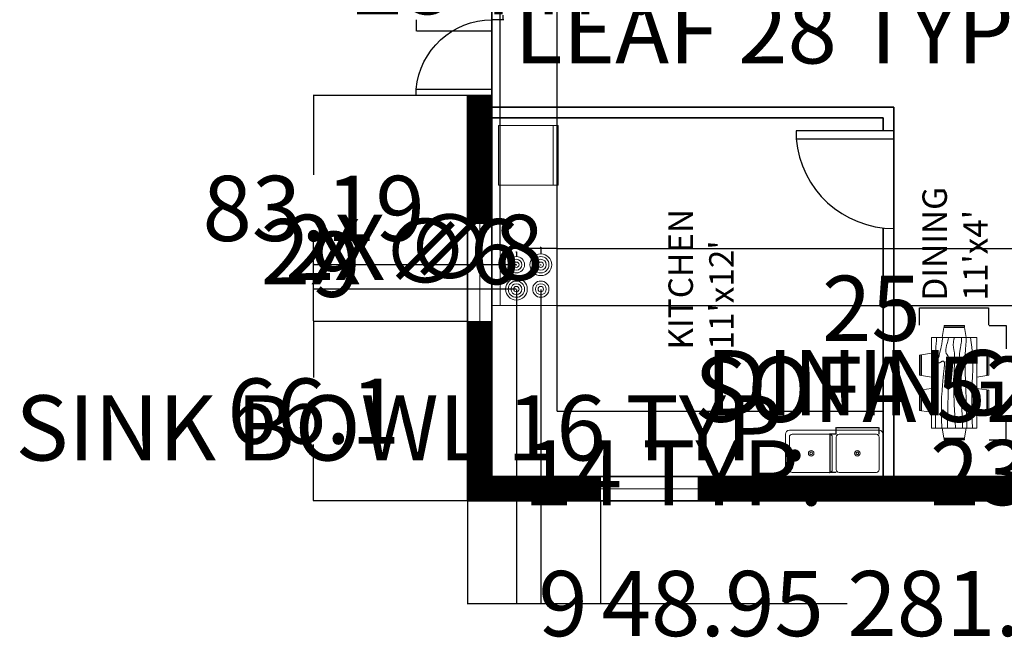
# Model space of a CAD drawing. Units: inches. Extents: x -1226 to 4538, y -998 to 1029.
# Tile 1 of 5: x -1226 to -864, y -998 to -767. Entities that reach past the tile are written whole.
import ezdxf

# ---------------------------------------------------------------- set-up
doc = ezdxf.new("R2010")
doc.units = ezdxf.units.IN
doc.header["$MEASUREMENT"] = 0
for name, color, linetype, lineweight in [('A-ANNO-DIMS', 2, 'Continuous', 18), ('A-AREA-IDEN', 7, 'Continuous', 18), ('A-DOOR', 4, 'Continuous', 25), ('A-EQPM', 8, 'Continuous', 18), ('A-FLOR-CASE', 8, 'Continuous', 25), ('A-FLOR-FIXT', 9, 'Continuous', 18), ('A-FURN', 8, 'Continuous', 18), ('A-GLAZ', 3, 'Continuous', 18), ('A-WALL', 7, 'Continuous', 35), ('A-WALL-PATT', 1, 'Continuous', 13)]:
    doc.layers.add(name, color=color, linetype=linetype, lineweight=lineweight)
doc.styles.get("Standard").update_dxf_attribs({"font": 'arial.ttf'})
doc.dimstyles.get("Standard").update_dxf_attribs({"dimtxt": 24, "dimasz": 0.18, "dimexe": 0.18, "dimexo": 0.0625, "dimgap": 0.09, "dimtad": 0, "dimtih": 1, "dimtoh": 1, "dimdec": 0, "dimzin": 0, "dimdsep": 46, "dimlunit": 4, "dimtxsty": 'Standard', "dimcen": 0.09, "dimadec": 0, "dimazin": 0, "dimtfac": 1, "dimtdec": 0, "dimtofl": 0, "dimtmove": 0, "dimatfit": 3, "dimfxl": 1, "dimtolj": 1, "dimtzin": 0, "dimarcsym": 0})

# ---------------------------------------------------------------- blocks, each defined once
blk = doc.blocks.new('Dining Set - 36 x 72 in.')
for p, q in [((-22.2343, 26.00059), (-23.4847, 17.99762)), ((-22.2304, 26), (-5.7608, 26)), ((-22, 27.5), (-22.1562, 26.50042)), ((-5.8416, 26.5), (-22.1534, 26.5)), ((-22, 27.5), (-6, 27.5)), ((-5.8437, 26.49966), (-6, 27.5)), ((-4.5152, 17.99762), (-5.7655, 25.99926)), ((5.7657, 26.00059), (4.5153, 17.99762)), ((5.7696, 26), (22.2392, 26)), ((6, 27.5), (5.8438, 26.50042)), ((22.1584, 26.5), (5.8466, 26.5)), ((6, 27.5), (22, 27.5)), ((22.1563, 26.49966), (22, 27.5)), ((23.4848, 17.99762), (22.2345, 25.99926)), ((36, 18), (-36, 18)), ((-36, 18), (-36, -18)), ((36, -18), (36, 18)), ((-45.5, 8), (-44.5004, 8.15617)), ((-45.5, 8), (-45.5, -8)), ((-44.5, -8.15843), (-44.5, 8.15338)), ((-44.0006, 8.23428), (-35.9976, 9.48474)), ((-44, 8.23041), (-44, -8.23915)), ((44.0006, 8.23428), (35.9976, 9.48474)), ((44, 8.23041), (44, -8.23915)), ((44.5, -8.15843), (44.5, 8.15338)), ((45.5, 8), (44.5005, 8.15617)), ((45.5, 8), (45.5, -8)), ((-44.4997, -8.15631), (-45.5, -8)), ((-35.9976, -9.48476), (-43.9993, -8.2345)), ((35.9976, -9.48476), (43.9993, -8.2345)), ((44.4997, -8.15631), (45.5, -8)), ((-36, -18), (36, -18)), ((-22.2343, -26.0006), (-23.4847, -17.99762)), ((-4.5152, -17.99762), (-5.7655, -25.99928)), ((5.7657, -26.0006), (4.5153, -17.99762)), ((23.4848, -17.99762), (22.2345, -25.99928)), ((-22.2304, -26), (-5.7608, -26)), ((-22, -27.5), (-22.1562, -26.50044)), ((-5.8416, -26.5), (-22.1534, -26.5)), ((-22, -27.5), (-6, -27.5)), ((-5.8437, -26.49967), (-6, -27.5)), ((5.7696, -26), (22.2392, -26)), ((6, -27.5), (5.8438, -26.50044)), ((22.1584, -26.5), (5.8466, -26.5)), ((6, -27.5), (22, -27.5)), ((22.1563, -26.49967), (22, -27.5))]:
    blk.add_line(p, q)
for points in [[(-36, 15), (-31.1772, 14.97754), (-26.8079, 14.91406), (-22.8538, 14.81543), (-19.276, 14.6875), (-16.0362, 14.53613), (-13.0957, 14.36718), (-10.4159, 14.18652), (-7.9583, 14), (-5.6904, 13.81315), (-3.6035, 13.63021), (-1.6954, 13.45508), (0.0365, 13.29166), (1.5945, 13.14388), (2.9811, 13.01562), (4.1988, 12.9108), (5.25, 12.83333), (6.1393, 12.78613), (6.8802, 12.76823), (7.4883, 12.77767), (7.9792, 12.8125), (8.3685, 12.87077), (8.6719, 12.95052), (8.9049, 13.0498), (9.0833, 13.16666), (9.2205, 13.29899), (9.3216, 13.44401), (9.3895, 13.59879), (9.4271, 13.76041), (9.4373, 13.92594), (9.4232, 14.09245), (9.3875, 14.257), (9.3333, 14.41666), (9.2638, 14.56917), (9.1836, 14.71484), (9.0975, 14.85465), (9.0104, 14.98958), (8.9272, 15.1206), (8.8529, 15.2487), (8.7922, 15.37483), (8.75, 15.5), (8.7305, 15.62467), (8.7344, 15.74739), (8.7617, 15.86621), (8.8125, 15.97916), (8.8867, 16.08431), (8.9844, 16.17968), (9.1055, 16.26334), (9.25, 16.33333), (9.4189, 16.38802), (9.6172, 16.42708), (9.8506, 16.45052), (10.125, 16.45833), (10.4463, 16.45052), (10.8203, 16.42708), (11.2529, 16.38802), (11.75, 16.33333), (12.3184, 16.26318), (12.9694, 16.17838), (13.7151, 16.07991), (14.5677, 15.96875), (15.5395, 15.84586), (16.6426, 15.71224), (17.8893, 15.56884), (19.2917, 15.41666), (20.859, 15.25667), (22.5879, 15.08984), (24.4721, 14.91715), (26.5052, 14.73958), (28.6809, 14.5581), (30.9929, 14.3737), (33.4347, 14.18733), (36, 14)], [(-36, 10), (-28.9766, 10.14274), (-23.1725, 10.20442), (-18.4241, 10.19775), (-14.5677, 10.13541), (-11.4399, 10.03011), (-8.877, 9.89453), (-6.7154, 9.74137), (-4.7917, 9.58333), (-2.9698, 9.43082), (-1.2246, 9.28515), (0.4415, 9.14534), (2.026, 9.01041), (3.5266, 8.87939), (4.9408, 8.7513), (6.266, 8.62516), (7.5, 8.5), (8.6411, 8.37549), (9.6914, 8.2539), (10.6538, 8.13818), (11.5312, 8.03125), (12.3267, 7.93603), (13.043, 7.85547), (13.6831, 7.79248), (14.25, 7.75), (14.7471, 7.7303), (15.1797, 7.73307), (15.5537, 7.75732), (15.875, 7.80208), (16.1494, 7.86637), (16.3828, 7.94922), (16.5811, 8.04964), (16.75, 8.16666), (16.8944, 8.29915), (17.0143, 8.44531), (17.1089, 8.60319), (17.1771, 8.77083), (17.218, 8.94629), (17.2305, 9.1276), (17.2137, 9.31282), (17.1667, 9.5), (17.0895, 9.6875), (16.987, 9.875), (16.8649, 10.0625), (16.7292, 10.25), (16.5856, 10.4375), (16.4401, 10.625), (16.2985, 10.8125), (16.1667, 11), (16.05, 11.18733), (15.9518, 11.3737), (15.8752, 11.5581), (15.8229, 11.73958), (15.798, 11.91715), (15.8034, 12.08984), (15.842, 12.25667), (15.9167, 12.41666), (16.0295, 12.56836), (16.1784, 12.70833), (16.3605, 12.83268), (16.5729, 12.9375), (16.8127, 13.01888), (17.0768, 13.07291), (17.3625, 13.0957), (17.6667, 13.08333), (17.9894, 13.03312), (18.3418, 12.94726), (18.7382, 12.82918), (19.1927, 12.68229), (19.7195, 12.51001), (20.3327, 12.31575), (21.0465, 12.10294), (21.875, 11.875), (22.8357, 11.63354), (23.959, 11.37304), (25.2786, 11.08618), (26.8282, 10.76562), (28.6414, 10.40405), (30.752, 9.99414), (33.1936, 9.52856), (36, 9)], [(-36, 5.5), (-30.7157, 5.3348), (-26.069, 5.20963), (-21.9946, 5.11767), (-18.4271, 5.05208), (-15.3009, 5.00602), (-12.5508, 4.97265), (-10.1112, 4.94515), (-7.9167, 4.91666), (-5.909, 4.88167), (-4.0586, 4.83984), (-2.3429, 4.79215), (-0.7396, 4.73958), (0.7739, 4.6831), (2.22, 4.6237), (3.6213, 4.56233), (5, 4.5), (6.373, 4.43782), (7.7344, 4.3776), (9.0723, 4.32129), (10.375, 4.27083), (11.6309, 4.22819), (12.8281, 4.19531), (13.9551, 4.17415), (15, 4.16666), (15.954, 4.17448), (16.819, 4.19791), (17.6001, 4.23698), (18.3021, 4.29166), (18.9299, 4.36198), (19.4883, 4.44791), (19.9823, 4.54948), (20.4167, 4.66666), (20.7969, 4.79899), (21.1302, 4.94401), (21.4245, 5.09879), (21.6875, 5.26041), (21.9271, 5.42594), (22.1511, 5.59245), (22.3672, 5.757), (22.5834, 5.91666), (22.8065, 6.06868), (23.0404, 6.21093), (23.2879, 6.34147), (23.5521, 6.45833), (23.8358, 6.55957), (24.142, 6.64323), (24.4735, 6.70735), (24.8334, 6.75), (25.2235, 6.76969), (25.642, 6.76692), (26.0858, 6.74267), (26.5521, 6.69791), (27.0379, 6.63362), (27.5404, 6.55078), (28.0565, 6.45036), (28.5834, 6.33333), (29.1242, 6.19987), (29.7071, 6.04687), (30.3661, 5.87044), (31.1354, 5.66666), (32.0493, 5.43164), (33.142, 5.16146), (34.4475, 4.85221), (36, 4.5)], [(-36, -1), (-30.7915, -0.6591), (-26.0195, -0.38216), (-21.6519, -0.16284), (-17.6563, 0.00521), (-14.0005, 0.12833), (-10.6523, 0.21289), (-7.5796, 0.26522), (-4.75, 0.29166), (-2.134, 0.29793), (0.2878, 0.28711), (2.5317, 0.26163), (4.6146, 0.22396), (6.5529, 0.17651), (8.3633, 0.12174), (10.0623, 0.06209), (11.6667, 0), (13.1899, -0.06201), (14.6341, -0.1211), (15.9982, -0.17432), (17.2813, -0.21875), (18.4823, -0.25147), (19.6003, -0.26953), (20.6343, -0.27002), (21.5834, -0.25), (22.4481, -0.20768), (23.2357, -0.14584), (23.9549, -0.06836), (24.6146, 0.02083), (25.2235, 0.11784), (25.7904, 0.21875), (26.3241, 0.31966), (26.8334, 0.41666), (27.3265, 0.50618), (27.8099, 0.58593), (28.2894, 0.65397), (28.7709, 0.70833), (29.2601, 0.74707), (29.763, 0.76823), (30.2855, 0.76985), (30.8334, 0.75), (31.4088, 0.70784), (31.9994, 0.64713), (32.589, 0.57275), (33.1615, 0.48958), (33.7008, 0.4025), (34.1908, 0.3164), (34.6153, 0.23616), (34.9584, 0.16666), (35.2099, 0.11165), (35.3848, 0.07031), (35.504, 0.04069), (35.5886, 0.02083), (35.6594, 0.00879), (35.7377, 0.0026), (35.8442, 0.00032), (36, 0)], [(-36, -6.5), (-27.1843, -6.31267), (-20.084, -6.1263), (-14.469, -5.9419), (-10.1094, -5.76042), (-6.7752, -5.58285), (-4.2363, -5.41016), (-2.2629, -5.24333), (-0.625, -5.08334), (0.8708, -4.93099), (2.2715, -4.78646), (3.5872, -4.64974), (4.8281, -4.52084), (6.0046, -4.39974), (7.127, -4.28646), (8.2053, -4.18099), (9.25, -4.08334), (10.2705, -3.99382), (11.2734, -3.91407), (12.2647, -3.84603), (13.25, -3.79167), (14.2354, -3.75293), (15.2266, -3.73177), (16.2295, -3.73015), (17.25, -3.75), (18.2912, -3.79248), (19.3451, -3.85547), (20.4009, -3.93604), (21.4479, -4.03125), (22.4754, -4.13819), (23.4727, -4.25391), (24.4289, -4.37549), (25.3334, -4.5), (26.1785, -4.62492), (26.9694, -4.74935), (27.7145, -4.87281), (28.4219, -4.99479), (29.1, -5.11483), (29.7572, -5.23242), (30.4016, -5.34709), (31.0417, -5.45834), (31.6837, -5.56437), (32.3262, -5.65821), (32.9658, -5.73153), (33.599, -5.77604), (34.2224, -5.78345), (34.8327, -5.74545), (35.4264, -5.65373), (36, -5.5)], [(-36, -10), (-26.4022, -9.81299), (-18.4675, -9.62891), (-11.9839, -9.45069), (-6.7396, -9.28125), (-2.5226, -9.12354), (0.8789, -8.98047), (3.6769, -8.85498), (6.0833, -8.75), (8.2767, -8.66765), (10.3021, -8.60677), (12.1712, -8.56543), (13.8958, -8.54167), (15.4876, -8.53353), (16.9583, -8.53907), (18.3197, -8.55632), (19.5834, -8.58334), (20.7616, -8.61841), (21.8685, -8.66081), (22.9188, -8.71004), (23.9271, -8.76563), (24.9081, -8.82707), (25.8763, -8.89388), (26.8465, -8.96558), (27.8334, -9.04167), (28.8474, -9.12118), (29.8828, -9.20117), (30.93, -9.27824), (31.9792, -9.34896), (33.0205, -9.40991), (34.0443, -9.45768), (35.0407, -9.48885), (36, -9.5)], [(-36, -14.5), (-30.0881, -14.33513), (-25.0332, -14.21224), (-20.7312, -14.12647), (-17.0781, -14.07292), (-13.97, -14.04671), (-11.3027, -14.04297), (-8.9724, -14.05681), (-6.875, -14.08334), (-4.9224, -14.11833), (-3.0905, -14.16016), (-1.3709, -14.20785), (0.2448, -14.26042), (1.7647, -14.3169), (3.1973, -14.3763), (4.5507, -14.43767), (5.8333, -14.5), (7.0554, -14.5621), (8.235, -14.62175), (9.3922, -14.67652), (10.5469, -14.72396), (11.7192, -14.76164), (12.929, -14.78711), (14.1965, -14.79794), (15.5417, -14.79167), (16.9933, -14.76424), (18.6152, -14.70508), (20.4804, -14.60197), (22.6615, -14.44271), (25.2312, -14.21509), (28.2624, -13.9069), (31.8277, -13.50594), (36, -13)]]:
    blk.add_lwpolyline(points)
blk = doc.blocks.new('DOOR-SWING-36')
for p, q in [((36, 36), (0, 36)), ((0, 36), (0, 33)), ((0, 33), (36, 33)), ((36, 33), (36, 36))]:
    blk.add_line(p, q)
blk.add_arc((36, 36.14), 36.14, 184.9791, 270)
blk = doc.blocks.new('DOOR-SWING-NARROW')
for p, q in [((27.84, 27.84), (0, 27.84)), ((0, 27.84), (0, 25.52)), ((0, 25.52), (27.84, 25.52)), ((27.84, 25.52), (27.84, 27.84))]:
    blk.add_line(p, q)
blk.add_arc((27.84, 27.94), 27.94, 184.9791, 270)
blk = doc.blocks.new('WIN-36')
for p, q in [((0, 36), (9, 36)), ((4.5, 0), (4.5, 36)), ((0, 0), (9, 0))]:
    blk.add_line(p, q)
blk = doc.blocks.new('SINK-BOWL-STANDARD')
blk.add_line((15.75, 1), (15.75, 13))
for points in [[(0, 1), (0, 13)], [(1, 14), (14.75, 14)], [(14.75, 0), (1, 0)]]:
    blk.add_lwpolyline(points)
for radius in [1, 0.5]:
    blk.add_circle((8, 7), radius)
for centre, start, end in [((1, 13), 90, 180), ((14.75, 13), 0, 90), ((1, 1), 180, 270), ((14.75, 1), 270, 0)]:
    blk.add_arc(centre, 1, start, end)
blk = doc.blocks.new('BURNER-6IN')
for radius in [3, 2, 1]:
    blk.add_circle((3, 3), radius)
blk = doc.blocks.new('BURNER-8IN')
for radius in [4, 3, 2, 1]:
    blk.add_circle((4, 4), radius)
blk = doc.blocks.new('*D28')
at = {"layer": 'A-ANNO-DIMS', "color": 0, "lineweight": -2, "transparency": 16777216}
for p, q in [((-1080.03, -767.33), (-1080.03, -771.62)), ((-1052.19, -767.33), (-1052.19, -771.62)), ((-1079.85, -771.44), (-1052.37, -771.44)), ((-1052.19, -771.44), (-1052.01, -771.44))]:
    blk.add_line(p, q, dxfattribs=at)
at = {"layer": 'A-ANNO-DIMS', "color": 0, "transparency": 16777216}
for points in [[(-1079.85, -771.41), (-1079.85, -771.47), (-1080.03, -771.44)], [(-1052.37, -771.41), (-1052.37, -771.47), (-1052.19, -771.44)]]:
    blk.add_solid(points, dxfattribs=at)
at = {"layer": 'Defpoints', "color": 0, "transparency": 16777216}
for p in [(-1080.03, -767.26), (-1052.19, -767.26), (-1052.19, -771.44)]:
    blk.add_point(p, dxfattribs=at)
at = {"layer": 'A-ANNO-DIMS', "color": 0, "transparency": 16777216, "insert": (-947.45, -771.44), "char_height": 24, "attachment_point": 5}
blk.add_mtext('\\A1;LEAF 28 TYP.', dxfattribs=at)
blk = doc.blocks.new('*D29')
at = {"layer": 'A-ANNO-DIMS', "color": 0, "lineweight": -2, "transparency": 16777216}
for p, q in [((-1052.13, -739.42), (-1047.83, -739.42)), ((-1048.01, -739.6), (-1048.01, -741)), ((-1052.13, -767.26), (-1047.83, -767.26)), ((-1048.01, -767.08), (-1048.01, -765.69))]:
    blk.add_line(p, q, dxfattribs=at)
at = {"layer": 'A-ANNO-DIMS', "color": 0, "transparency": 16777216}
for points in [[(-1048.04, -739.6), (-1047.98, -739.6), (-1048.01, -739.42)], [(-1048.04, -767.08), (-1047.98, -767.08), (-1048.01, -767.26)]]:
    blk.add_solid(points, dxfattribs=at)
at = {"layer": 'Defpoints', "color": 0, "transparency": 16777216}
for p in [(-1052.19, -739.42), (-1048.01, -739.42), (-1052.19, -767.26)]:
    blk.add_point(p, dxfattribs=at)
at = {"layer": 'A-ANNO-DIMS', "color": 0, "transparency": 16777216, "insert": (-1048.01, -753.34), "char_height": 24, "attachment_point": 5}
blk.add_mtext('\\A1;28 TYP.', dxfattribs=at)
blk = doc.blocks.new('*D34')
at = {"layer": 'A-ANNO-DIMS', "color": 0, "lineweight": -2, "transparency": 16777216}
for p, q in [((-768.95, -903.42), (-769.13, -903.42)), ((-768.95, -911.16), (-768.95, -903.24)), ((-717.1, -903.42), (-768.77, -903.42)), ((-716.92, -911.16), (-716.92, -903.24))]:
    blk.add_line(p, q, dxfattribs=at)
at = {"layer": 'A-ANNO-DIMS', "color": 0, "transparency": 16777216}
for points in [[(-768.77, -903.39), (-768.77, -903.45), (-768.95, -903.42)], [(-717.1, -903.39), (-717.1, -903.45), (-716.92, -903.42)]]:
    blk.add_solid(points, dxfattribs=at)
at = {"layer": 'Defpoints', "color": 0, "transparency": 16777216}
for p in [(-768.95, -903.42), (-768.95, -911.22), (-716.92, -911.22)]:
    blk.add_point(p, dxfattribs=at)
at = {"layer": 'A-ANNO-DIMS', "color": 0, "transparency": 16777216, "insert": (-877.88, -903.42), "char_height": 24, "attachment_point": 5}
blk.add_mtext('\\A1;SOFA 52 TYP.', dxfattribs=at)
blk = doc.blocks.new('*D35')
at = {"layer": 'A-ANNO-DIMS', "color": 0, "lineweight": -2, "transparency": 16777216}
for p, q in [((-769.01, -911.22), (-776.94, -911.22)), ((-776.76, -911.4), (-776.76, -933.75)), ((-769.01, -933.93), (-776.94, -933.93)), ((-776.76, -934.11), (-776.94, -934.11)), ((-776.76, -933.93), (-776.76, -934.11))]:
    blk.add_line(p, q, dxfattribs=at)
at = {"layer": 'A-ANNO-DIMS', "color": 0, "transparency": 16777216}
for points in [[(-776.79, -911.4), (-776.73, -911.4), (-776.76, -911.22)], [(-776.79, -933.75), (-776.73, -933.75), (-776.76, -933.93)]]:
    blk.add_solid(points, dxfattribs=at)
at = {"layer": 'Defpoints', "color": 0, "transparency": 16777216}
for p in [(-768.95, -911.22), (-776.76, -933.93), (-768.95, -933.93)]:
    blk.add_point(p, dxfattribs=at)
at = {"layer": 'A-ANNO-DIMS', "color": 0, "transparency": 16777216, "insert": (-835.64, -934.11), "char_height": 24, "attachment_point": 5}
blk.add_mtext('\\A1;23 TYP.', dxfattribs=at)
blk = doc.blocks.new('*D40')
at = {"layer": 'A-ANNO-DIMS', "color": 0, "lineweight": -2, "transparency": 16777216}
for p, q in [((-925.4, -917.65), (-925.58, -917.65)), ((-925.4, -919.95), (-925.4, -917.47)), ((-909.83, -917.65), (-925.22, -917.65)), ((-909.65, -919.95), (-909.65, -917.47))]:
    blk.add_line(p, q, dxfattribs=at)
at = {"layer": 'A-ANNO-DIMS', "color": 0, "transparency": 16777216}
for points in [[(-925.22, -917.62), (-925.22, -917.68), (-925.4, -917.65)], [(-909.83, -917.62), (-909.83, -917.68), (-909.65, -917.65)]]:
    blk.add_solid(points, dxfattribs=at)
at = {"layer": 'Defpoints', "color": 0, "transparency": 16777216}
for p in [(-925.4, -917.65), (-925.4, -920.02), (-909.65, -920.02)]:
    blk.add_point(p, dxfattribs=at)
at = {"layer": 'A-ANNO-DIMS', "color": 0, "transparency": 16777216, "insert": (-1081.83, -917.65), "char_height": 24, "attachment_point": 5}
blk.add_mtext('\\A1;SINK BOWL 16 TYP.', dxfattribs=at)
blk = doc.blocks.new('*D41')
at = {"layer": 'A-ANNO-DIMS', "color": 0, "lineweight": -2, "transparency": 16777216}
for p, q in [((-925.46, -920.02), (-927.94, -920.02)), ((-927.76, -920.2), (-927.76, -933.84)), ((-925.46, -934.02), (-927.94, -934.02)), ((-927.76, -934.2), (-927.94, -934.2)), ((-927.76, -934.02), (-927.76, -934.2))]:
    blk.add_line(p, q, dxfattribs=at)
at = {"layer": 'A-ANNO-DIMS', "color": 0, "transparency": 16777216}
for points in [[(-927.79, -920.2), (-927.73, -920.2), (-927.76, -920.02)], [(-927.79, -933.84), (-927.73, -933.84), (-927.76, -934.02)]]:
    blk.add_solid(points, dxfattribs=at)
at = {"layer": 'Defpoints', "color": 0, "transparency": 16777216}
for p in [(-925.4, -920.02), (-927.76, -934.02), (-925.4, -934.02)]:
    blk.add_point(p, dxfattribs=at)
at = {"layer": 'A-ANNO-DIMS', "color": 0, "transparency": 16777216, "insert": (-985.31, -934.2), "char_height": 24, "attachment_point": 5}
blk.add_mtext('\\A1;14 TYP.', dxfattribs=at)
blk = doc.blocks.new('*D46')
at = {"layer": 'A-ANNO-DIMS', "color": 0, "lineweight": -2, "transparency": 16777216}
for p, q in [((-869.17, -879.93), (-862.73, -879.93)), ((-862.91, -880.11), (-862.91, -888.51)), ((-862.91, -921.91), (-862.91, -913.51)), ((-869.17, -922.09), (-862.73, -922.09))]:
    blk.add_line(p, q, dxfattribs=at)
at = {"layer": 'A-ANNO-DIMS', "color": 0, "transparency": 16777216}
for points in [[(-862.94, -880.11), (-862.88, -880.11), (-862.91, -879.93)], [(-862.94, -921.91), (-862.88, -921.91), (-862.91, -922.09)]]:
    blk.add_solid(points, dxfattribs=at)
at = {"layer": 'Defpoints', "color": 0, "transparency": 16777216}
for p in [(-869.23, -879.93), (-862.91, -879.93), (-869.23, -922.09)]:
    blk.add_point(p, dxfattribs=at)
at = {"layer": 'A-ANNO-DIMS', "color": 0, "transparency": 16777216, "insert": (-862.91, -901.01), "char_height": 24, "attachment_point": 5}
blk.add_mtext('\\A1;DINING SET 42', dxfattribs=at)
blk = doc.blocks.new('*D47')
at = {"layer": 'A-ANNO-DIMS', "color": 0, "lineweight": -2, "transparency": 16777216}
for p, q in [((-894.72, -879.87), (-894.72, -873.43)), ((-869.23, -879.87), (-869.23, -873.43)), ((-894.72, -873.61), (-894.9, -873.61)), ((-869.41, -873.61), (-894.54, -873.61))]:
    blk.add_line(p, q, dxfattribs=at)
at = {"layer": 'A-ANNO-DIMS', "color": 0, "transparency": 16777216}
for points in [[(-894.54, -873.58), (-894.54, -873.64), (-894.72, -873.61)], [(-869.41, -873.58), (-869.41, -873.64), (-869.23, -873.61)]]:
    blk.add_solid(points, dxfattribs=at)
at = {"layer": 'Defpoints', "color": 0, "transparency": 16777216}
for p in [(-894.72, -873.61), (-894.72, -879.93), (-869.23, -879.93)]:
    blk.add_point(p, dxfattribs=at)
at = {"layer": 'A-ANNO-DIMS', "color": 0, "transparency": 16777216, "insert": (-912.47, -873.61), "char_height": 24, "attachment_point": 5}
blk.add_mtext('\\A1;25', dxfattribs=at)
blk = doc.blocks.new('*D56')
at = {"layer": 'A-ANNO-DIMS', "color": 0, "lineweight": -2, "transparency": 16777216}
for p, q in [((-1061.17, -944.59), (-1061.17, -982.51)), ((-1012.21, -944.64), (-1012.21, -982.51)), ((-1060.99, -982.33), (-1012.39, -982.33)), ((-1012.21, -982.33), (-1012.03, -982.33))]:
    blk.add_line(p, q, dxfattribs=at)
at = {"layer": 'A-ANNO-DIMS', "color": 0, "transparency": 16777216}
for points in [[(-1060.99, -982.3), (-1060.99, -982.36), (-1061.17, -982.33)], [(-1012.39, -982.3), (-1012.39, -982.36), (-1012.21, -982.33)]]:
    blk.add_solid(points, dxfattribs=at)
at = {"layer": 'Defpoints', "color": 0, "transparency": 16777216}
for p in [(-1061.17, -944.53), (-1012.21, -944.57), (-1012.21, -982.33)]:
    blk.add_point(p, dxfattribs=at)
at = {"layer": 'A-ANNO-DIMS', "color": 0, "transparency": 16777216, "insert": (-970.88, -982.33), "char_height": 24, "attachment_point": 5}
blk.add_mtext('\\A1;48.95', dxfattribs=at)
blk = doc.blocks.new('*D57')
at = {"layer": 'A-ANNO-DIMS', "color": 0, "lineweight": -2, "transparency": 16777216}
for p, q in [((-1012.21, -944.64), (-1012.21, -982.51)), ((-730.47, -944.64), (-730.47, -982.51)), ((-1012.03, -982.33), (-921.41, -982.33)), ((-730.65, -982.33), (-821.28, -982.33))]:
    blk.add_line(p, q, dxfattribs=at)
at = {"layer": 'A-ANNO-DIMS', "color": 0, "transparency": 16777216}
for points in [[(-1012.03, -982.3), (-1012.03, -982.36), (-1012.21, -982.33)], [(-730.65, -982.3), (-730.65, -982.36), (-730.47, -982.33)]]:
    blk.add_solid(points, dxfattribs=at)
at = {"layer": 'Defpoints', "color": 0, "transparency": 16777216}
for p in [(-1012.21, -944.57), (-730.47, -944.58), (-730.47, -982.33)]:
    blk.add_point(p, dxfattribs=at)
at = {"layer": 'A-ANNO-DIMS', "color": 0, "transparency": 16777216, "insert": (-871.34, -982.33), "char_height": 24, "attachment_point": 5}
blk.add_mtext('\\A1;281.74', dxfattribs=at)
blk = doc.blocks.new('*D59')
at = {"layer": 'A-ANNO-DIMS', "color": 0, "lineweight": -2, "transparency": 16777216}
for p, q in [((-1061.14, -878.43), (-1117.96, -878.43)), ((-1117.78, -878.61), (-1117.78, -899.13)), ((-1117.78, -944.35), (-1117.78, -923.82)), ((-1061.23, -944.53), (-1117.96, -944.53))]:
    blk.add_line(p, q, dxfattribs=at)
at = {"layer": 'A-ANNO-DIMS', "color": 0, "transparency": 16777216}
for points in [[(-1117.81, -878.61), (-1117.75, -878.61), (-1117.78, -878.43)], [(-1117.81, -944.35), (-1117.75, -944.35), (-1117.78, -944.53)]]:
    blk.add_solid(points, dxfattribs=at)
at = {"layer": 'Defpoints', "color": 0, "transparency": 16777216}
for p in [(-1117.78, -878.43), (-1061.07, -878.43), (-1061.17, -944.53)]:
    blk.add_point(p, dxfattribs=at)
at = {"layer": 'A-ANNO-DIMS', "color": 0, "transparency": 16777216, "insert": (-1117.78, -911.48), "char_height": 24, "attachment_point": 5}
blk.add_mtext('\\A1;66.1', dxfattribs=at)
blk = doc.blocks.new('*D60')
at = {"layer": 'A-ANNO-DIMS', "color": 0, "lineweight": -2, "transparency": 16777216}
for p, q in [((-1061.23, -795.24), (-1117.96, -795.24)), ((-1117.78, -795.42), (-1117.78, -824.48)), ((-1117.78, -878.25), (-1117.78, -849.19)), ((-1061.14, -878.43), (-1117.96, -878.43))]:
    blk.add_line(p, q, dxfattribs=at)
at = {"layer": 'A-ANNO-DIMS', "color": 0, "transparency": 16777216}
for points in [[(-1117.81, -795.42), (-1117.75, -795.42), (-1117.78, -795.24)], [(-1117.81, -878.25), (-1117.75, -878.25), (-1117.78, -878.43)]]:
    blk.add_solid(points, dxfattribs=at)
at = {"layer": 'Defpoints', "color": 0, "transparency": 16777216}
for p in [(-1117.78, -795.24), (-1061.17, -795.24), (-1061.07, -878.43)]:
    blk.add_point(p, dxfattribs=at)
at = {"layer": 'A-ANNO-DIMS', "color": 0, "transparency": 16777216, "insert": (-1117.78, -836.83), "char_height": 24, "attachment_point": 5}
blk.add_mtext('\\A1;83.19', dxfattribs=at)
blk = doc.blocks.new('*D77')
at = {"layer": 'A-ANNO-DIMS', "color": 0, "lineweight": -2, "transparency": 16777216}
for p, q in [((-1049.16, -851.5), (-1049.16, -546.6)), ((-1048.98, -546.78), (-1028.34, -546.78)), ((-1028.16, -851.5), (-1028.16, -546.6)), ((-1028.16, -546.78), (-1027.98, -546.78))]:
    blk.add_line(p, q, dxfattribs=at)
at = {"layer": 'A-ANNO-DIMS', "color": 0, "transparency": 16777216}
for points in [[(-1048.98, -546.75), (-1048.98, -546.81), (-1049.16, -546.78)], [(-1028.34, -546.75), (-1028.34, -546.81), (-1028.16, -546.78)]]:
    blk.add_solid(points, dxfattribs=at)
at = {"layer": 'Defpoints', "color": 0, "transparency": 16777216}
for p in [(-1028.16, -546.78), (-1049.16, -851.56), (-1028.16, -851.56)]:
    blk.add_point(p, dxfattribs=at)
at = {"layer": 'A-ANNO-DIMS', "color": 0, "transparency": 16777216, "insert": (-1012.81, -546.78), "char_height": 24, "attachment_point": 5}
blk.add_mtext('\\A1;21', dxfattribs=at)
blk = doc.blocks.new('*D78')
at = {"layer": 'A-ANNO-DIMS', "color": 0, "lineweight": -2, "transparency": 16777216}
for p, q in [((-1028.09, -851.56), (-401.24, -851.56)), ((-401.42, -851.74), (-401.42, -872.38)), ((-1028.09, -872.56), (-401.24, -872.56)), ((-401.42, -872.74), (-401.6, -872.74)), ((-401.42, -872.56), (-401.42, -872.74))]:
    blk.add_line(p, q, dxfattribs=at)
at = {"layer": 'A-ANNO-DIMS', "color": 0, "transparency": 16777216}
for points in [[(-401.45, -851.74), (-401.39, -851.74), (-401.42, -851.56)], [(-401.45, -872.38), (-401.39, -872.38), (-401.42, -872.56)]]:
    blk.add_solid(points, dxfattribs=at)
at = {"layer": 'Defpoints', "color": 0, "transparency": 16777216}
for p in [(-1028.16, -851.56), (-1028.16, -872.56), (-401.42, -872.56)]:
    blk.add_point(p, dxfattribs=at)
at = {"layer": 'A-ANNO-DIMS', "color": 0, "transparency": 16777216, "insert": (-416.76, -872.74), "char_height": 24, "attachment_point": 5}
blk.add_mtext('\\A1;21', dxfattribs=at)
blk = doc.blocks.new('*D79')
at = {"layer": 'A-ANNO-DIMS', "color": 0, "lineweight": -2, "transparency": 16777216}
for p, q in [((-1043.16, -866.63), (-1043.16, -982.51)), ((-1034.16, -866.63), (-1034.16, -982.51)), ((-1042.98, -982.33), (-1034.34, -982.33)), ((-1034.16, -982.33), (-1033.98, -982.33))]:
    blk.add_line(p, q, dxfattribs=at)
at = {"layer": 'A-ANNO-DIMS', "color": 0, "transparency": 16777216}
for points in [[(-1042.98, -982.3), (-1042.98, -982.36), (-1043.16, -982.33)], [(-1034.34, -982.3), (-1034.34, -982.36), (-1034.16, -982.33)]]:
    blk.add_solid(points, dxfattribs=at)
at = {"layer": 'Defpoints', "color": 0, "transparency": 16777216}
for p in [(-1043.16, -866.56), (-1034.16, -866.56), (-1034.16, -982.33)]:
    blk.add_point(p, dxfattribs=at)
at = {"layer": 'A-ANNO-DIMS', "color": 0, "transparency": 16777216, "insert": (-1026, -982.33), "char_height": 24, "attachment_point": 5}
blk.add_mtext('\\A1;9', dxfattribs=at)
blk = doc.blocks.new('*D80')
at = {"layer": 'A-ANNO-DIMS', "color": 0, "lineweight": -2, "transparency": 16777216}
for p, q in [((-1043.22, -857.56), (-1117.96, -857.56)), ((-1117.78, -857.56), (-1117.78, -857.38)), ((-1117.78, -857.38), (-1117.6, -857.38)), ((-1117.78, -866.38), (-1117.78, -857.74)), ((-1043.22, -866.56), (-1117.96, -866.56))]:
    blk.add_line(p, q, dxfattribs=at)
at = {"layer": 'A-ANNO-DIMS', "color": 0, "transparency": 16777216}
for points in [[(-1117.81, -857.74), (-1117.75, -857.74), (-1117.78, -857.56)], [(-1117.81, -866.38), (-1117.75, -866.38), (-1117.78, -866.56)]]:
    blk.add_solid(points, dxfattribs=at)
at = {"layer": 'Defpoints', "color": 0, "transparency": 16777216}
for p in [(-1117.78, -857.56), (-1043.16, -857.56), (-1043.16, -866.56)]:
    blk.add_point(p, dxfattribs=at)
at = {"layer": 'A-ANNO-DIMS', "color": 0, "transparency": 16777216, "insert": (-1109.62, -857.38), "char_height": 24, "attachment_point": 5}
blk.add_mtext('\\A1;9', dxfattribs=at)
blk = doc.blocks.new('*D81')
at = {"layer": 'A-ANNO-DIMS', "color": 0, "lineweight": -2, "transparency": 16777216}
for p, q in [((-1043.34, -852.76), (-1043.16, -852.76)), ((-1043.16, -852.76), (-1043.16, -854.38)), ((-1043.25, -857.56), (-1043.07, -857.56)), ((-1043.16, -857.65), (-1043.16, -857.47))]:
    blk.add_line(p, q, dxfattribs=at)
at = {"layer": 'A-ANNO-DIMS', "color": 0, "transparency": 16777216}
blk.add_solid([(-1043.13, -854.38), (-1043.19, -854.38), (-1043.16, -854.56)], dxfattribs=at)
at = {"layer": 'Defpoints', "color": 0, "transparency": 16777216}
for p in [(-1043.16, -854.56), (-1043.15, -860.56)]:
    blk.add_point(p, dxfattribs=at)
at = {"layer": 'A-ANNO-DIMS', "color": 0, "transparency": 16777216, "insert": (-1089.7, -852.76), "char_height": 24, "attachment_point": 5}
blk.add_mtext('\\A1;2X ∅6', dxfattribs=at)
blk = doc.blocks.new('*D82')
at = {"layer": 'A-ANNO-DIMS', "color": 0, "lineweight": -2, "transparency": 16777216}
for p, q in [((-1034.34, -851.16), (-1034.16, -851.16)), ((-1034.16, -851.16), (-1034.16, -853.38)), ((-1034.25, -857.56), (-1034.07, -857.56)), ((-1034.16, -857.65), (-1034.16, -857.47))]:
    blk.add_line(p, q, dxfattribs=at)
at = {"layer": 'A-ANNO-DIMS', "color": 0, "transparency": 16777216}
blk.add_solid([(-1034.13, -853.38), (-1034.19, -853.38), (-1034.16, -853.56)], dxfattribs=at)
at = {"layer": 'Defpoints', "color": 0, "transparency": 16777216}
for p in [(-1034.16, -853.56), (-1034.15, -861.56)]:
    blk.add_point(p, dxfattribs=at)
at = {"layer": 'A-ANNO-DIMS', "color": 0, "transparency": 16777216, "insert": (-1080.73, -851.16), "char_height": 24, "attachment_point": 5}
blk.add_mtext('\\A1;2X ∅8', dxfattribs=at)

msp = doc.modelspace()

# ---------------------------------------------------------------- hatches: boundary and pattern name
at = {"layer": 'A-WALL-PATT'}
h = msp.add_hatch(dxfattribs=at)
h.set_pattern_fill('ANSI31', color=256, angle=90)
h.set_pattern_definition([(135, (-1048.80633, 527.86775), (-0.088388348, -0.088388348), [])])
h.paths.add_polyline_path([(-1052.1662, -935.5274), (-1052.1662, -878.4295), (-1061.1662, -878.4295), (-1061.1662, -944.5274), (-1012.2132, -944.5274), (-1012.2132, -935.5274)])
h.paths.add_polyline_path([(-976.2132, -935.5274), (-976.2132, -944.5274), (-730.4734, -944.5274), (-730.4734, -935.5274)])
h.paths.add_polyline_path([(-694.4734, -935.5274), (-694.4734, -944.5274), (-651.0832, -944.5274), (-651.0832, -935.5274)])
h.paths.add_polyline_path([(-615.0832, -935.5274), (-615.0832, -944.5274), (-561.1662, -944.5274), (-561.1662, -935.5274)])
h.paths.add_polyline_path([(-712.9165, -584.5274), (-712.9165, -593.5274), (-657.3138, -593.5274), (-657.3138, -593.4838), (-597.3139, -593.4838), (-448.1662, -593.5274), (-448.1662, -713.5274), (-448.1662, -779.5274), (-439.1662, -779.5274), (-439.1662, -584.5274)])
h.paths.add_polyline_path([(-875.9292, -584.5274), (-875.9292, -593.5274), (-736.9165, -593.5274), (-736.9165, -584.5274)])
h.paths.add_polyline_path([(-950.5052, -584.5274), (-950.5052, -593.5274), (-911.9292, -593.5274), (-911.9292, -584.5274)])
h.paths.add_polyline_path([(-1011.0429, -584.5274), (-1011.0429, -593.5274), (-974.5052, -593.5274), (-974.5052, -584.5274)])
h.paths.add_polyline_path([(-1061.1662, -584.5274), (-1061.1662, -693.4459), (-1052.1662, -693.4459), (-1052.1662, -593.5274), (-1035.0429, -593.5274), (-1035.0429, -584.5274)])
h.paths.add_polyline_path([(-1061.1662, -795.2404), (-1061.1662, -842.4295), (-1052.1662, -842.4295), (-1052.1662, -795.2404)])
h.paths.add_polyline_path([(-1061.1662, -717.4459), (-1061.1662, -739.4249), (-1052.1662, -739.4249), (-1052.1662, -717.4459)])

# ---------------------------------------------------------------- linework, layer by layer
at = {"layer": 'A-EQPM'}
for p, q in [((-1049.7172, -828.3297), (-1049.7172, -806.3328)), ((-1049.7172, -806.3328), (-1027.7203, -806.3328)), ((-1029.5534, -828.3297), (-1029.5534, -806.3328)), ((-1027.7203, -806.3328), (-1027.7203, -828.3297)), ((-1049.7172, -828.3297), (-1029.5534, -828.3297)), ((-1027.7203, -828.3297), (-1029.5534, -828.3297)), ((-1049.1562, -872.5639), (-1049.1562, -851.5639))]:
    msp.add_line(p, q, dxfattribs=at)
msp.add_lwpolyline([(-1028.1562, -872.5639), (-1052.1562, -872.5639), (-1052.1562, -851.5639), (-1028.1562, -851.5639)], close=True, dxfattribs=at)
at = {"layer": 'A-FLOR-CASE'}
for p, q in [((-1052.1662, -851.5274), (-1028.1662, -851.5274)), ((-1028.1662, -911.5274), (-1028.1662, -851.5274)), ((-1028.1662, -911.5274), (-908.1662, -911.5274))]:
    msp.add_line(p, q, dxfattribs=at)
at = {"layer": 'A-FLOR-FIXT'}
msp.add_line((-908.1482, -935.5168), (-944.1482, -935.5168), dxfattribs=at)
for points in [[(-944.1482, -935.5168), (-944.1482, -920.0168)], [(-942.6482, -918.5168), (-909.6482, -918.5168)], [(-908.1482, -920.0168), (-908.1482, -935.5168)]]:
    msp.add_lwpolyline(points, dxfattribs=at)
for centre, start, end in [((-942.6482, -920.0168), 90, 180), ((-909.6482, -920.0168), 0, 90)]:
    msp.add_arc(centre, 1.5, start, end, dxfattribs=at)
at = {"layer": 'A-WALL'}
for p, q in [((-1052.1662, -935.5274), (-1052.1662, -593.5274)), ((-1061.1662, -944.5274), (-1061.1662, -795.2404)), ((-1052.1662, -799.5274), (-904.1662, -799.5274)), ((-904.1662, -935.5274), (-904.1662, -799.5274)), ((-1052.1662, -803.5274), (-908.1662, -803.5274)), ((-908.1662, -808.2178), (-908.1662, -803.5274)), ((-908.1662, -935.5274), (-908.1662, -843.9961)), ((-1052.1662, -935.5274), (-439.1662, -935.5274)), ((-1061.1662, -944.5274), (-561.1662, -944.5274))]:
    msp.add_line(p, q, dxfattribs=at)

# ---------------------------------------------------------------- block references
at = {"layer": 'A-DOOR', "extrusion": (0, 0, -1), "zscale": -1, "rotation": 180}
msp.add_blockref('DOOR-SWING-NARROW', (1080.027, -767.4013), dxfattribs=at)
at = {"layer": 'A-DOOR'}
msp.add_blockref('DOOR-SWING-36', (-940.169, -844.218), dxfattribs=at)
at = {"layer": 'A-EQPM'}
for name, p in [('BURNER-6IN', (-1046.156, -860.564)), ('BURNER-8IN', (-1038.156, -861.564))]:
    msp.add_blockref(name, p, dxfattribs=at)
for name, p, rotation in [('BURNER-8IN', (-1043.1564, -860.9071), 225), ('BURNER-6IN', (-1031.1564, -863.5638), 180)]:
    msp.add_blockref(name, p, dxfattribs=dict(at, rotation=rotation))
at = {"layer": 'A-FLOR-FIXT'}
msp.add_blockref('SINK-BOWL-STANDARD', (-942.648, -934.017), dxfattribs=at)
at = {"layer": 'A-FLOR-FIXT', "rotation": 180}
msp.add_blockref('SINK-BOWL-STANDARD', (-909.6483, -920.0167), dxfattribs=at)
at = {"layer": 'A-FURN', "xscale": 0.4633040936325969, "yscale": 0.4633040936325969, "zscale": 0.4633040936325969, "rotation": 90}
msp.add_blockref('Dining Set - 36 x 72 in.', (-881.9744, -901.0106), dxfattribs=at)
at = {"layer": 'A-GLAZ'}
msp.add_blockref('WIN-36', (-1061.073, -878.429), dxfattribs=at)
at = {"layer": 'A-GLAZ', "rotation": 270}
msp.add_blockref('WIN-36', (-1012.2127, -935.5741), dxfattribs=at)

# ---------------------------------------------------------------- texts
at = {"layer": 'A-AREA-IDEN', "char_height": 9, "attachment_point": 1, "rotation": 90}
for s, width, insert in [("DINING\\P11'x4'", 76.603238, (-893.6855, -870.7806)), ("KITCHEN\\P11'x12'", 52.541237, (-987.177, -888.7987))]:
    msp.add_mtext_dynamic_manual_height_columns(s, width=width, gutter_width=1, heights=[0], dxfattribs=dict(at, insert=insert))

# ---------------------------------------------------------------- dimensions: what is measured, and where the dimension line sits
at = {"layer": 'A-ANNO-DIMS'}
for base, p1, p2, override, picture, middle in [((-1028.1562, -546.7774), (-1049.1562, -851.5639), (-1028.1562, -851.5639), {"dimdec": 0, "dimlfac": 1, "dimrnd": 0, "dimzin": 0, "dimdsep": 46, "dimlunit": 2}, '*D77', (-1012.8084, -546.7774)), ((-1034.1562, -982.3314), (-1043.1562, -866.5639), (-1034.1562, -866.5639), {"dimdec": 0, "dimlfac": 1, "dimrnd": 0, "dimzin": 0, "dimdsep": 46, "dimlunit": 2}, '*D79', (-1025.9953, -982.3314)), ((-1012.2132, -982.3314), (-1061.1662, -944.5274), (-1012.2132, -944.5741), {"dimdec": 2, "dimlfac": 1, "dimrnd": 0, "dimzin": 0, "dimdsep": 46, "dimlunit": 2}, '*D56', (-970.8763, -982.3314)), ((-730.4734, -982.3314), (-1012.2132, -944.5741), (-730.4734, -944.5814), {"dimdec": 2, "dimlfac": 1, "dimrnd": 0, "dimzin": 0, "dimdsep": 46, "dimlunit": 2}, '*D57', (-871.3433, -982.3314))]:
    dim = msp.add_linear_dim(base=base, p1=p1, p2=p2, dimstyle='Standard', override=override, dxfattribs=at)
    dim.commit()
    dim.dimension.update_dxf_attribs({"geometry": picture, "text_midpoint": middle})
for base, p1, p2, angle, text, picture, middle in [((-1048.0119, -739.4249), (-1052.1878, -767.2643), (-1052.1878, -739.4249), 90, '<> TYP.', '*D29', (-1048.0119, -753.3446)), ((-925.3982, -917.6543), (-909.6482, -920.0168), (-925.3982, -920.0168), 180, 'SINK BOWL <> TYP.', '*D40', (-1081.8319, -917.6543)), ((-768.9517, -903.4189), (-716.9223, -911.2233), (-768.9517, -911.2233), 180, 'SOFA <> TYP.', '*D34', (-877.8765, -903.4189)), ((-862.9094, -879.9303), (-869.2335, -922.091), (-869.2335, -879.9303), 90, 'DINING SET <>', '*D46', (-862.9094, -901.0106)), ((-927.7607, -934.0168), (-925.3982, -920.0168), (-925.3982, -934.0168), 270, '<> TYP.', '*D41', (-985.3131, -934.1968)), ((-776.7561, -933.9346), (-768.9517, -911.2233), (-768.9517, -933.9346), 270, '<> TYP.', '*D35', (-835.6427, -934.1146))]:
    dim = msp.add_linear_dim(base=base, p1=p1, p2=p2, angle=angle, text=text, dimstyle='Standard', override={"dimdec": 0, "dimlfac": 1, "dimrnd": 0, "dimzin": 0, "dimdsep": 46, "dimlunit": 2}, dxfattribs=at)
    dim.commit()
    dim.dimension.update_dxf_attribs({"geometry": picture, "text_midpoint": middle})
dim = msp.add_linear_dim(base=(-1052.1878, -771.4403), p1=(-1080.0272, -767.2643), p2=(-1052.1878, -767.2643), text='LEAF <> TYP.', dimstyle='Standard', override={"dimdec": 0, "dimlfac": 1, "dimrnd": 0, "dimzin": 0, "dimdsep": 46, "dimlunit": 2}, dxfattribs=at)
dim.commit()
dim.dimension.update_dxf_attribs({"geometry": '*D28', "text_midpoint": (-947.4539, -771.4403)})
for base, p1, p2, angle, override, picture, middle in [((-1117.7772, -795.2404), (-1061.073, -878.4295), (-1061.1662, -795.2404), 90, {"dimdec": 2, "dimlfac": 1, "dimrnd": 0, "dimzin": 0, "dimdsep": 46, "dimlunit": 2}, '*D60', (-1117.7772, -836.8349)), ((-1117.7772, -857.5639), (-1043.1562, -866.5639), (-1043.1562, -857.5639), 90, {"dimdec": 0, "dimlfac": 1, "dimrnd": 0, "dimzin": 0, "dimdsep": 46, "dimlunit": 2}, '*D80', (-1109.6163, -857.3839)), ((-401.4162, -872.5639), (-1028.1562, -851.5639), (-1028.1562, -872.5639), 90, {"dimdec": 0, "dimlfac": 1, "dimrnd": 0, "dimzin": 0, "dimdsep": 46, "dimlunit": 2}, '*D78', (-416.7639, -872.7439)), ((-894.7152, -873.6062), (-869.2335, -879.9303), (-894.7152, -879.9303), 180, {"dimdec": 0, "dimlfac": 1, "dimrnd": 0, "dimzin": 0, "dimdsep": 46, "dimlunit": 2}, '*D47', (-912.4696, -873.6062)), ((-1117.7772, -878.4295), (-1061.1662, -944.5274), (-1061.073, -878.4295), 90, {"dimdec": 1, "dimlfac": 1, "dimrnd": 0, "dimzin": 0, "dimdsep": 46, "dimlunit": 2}, '*D59', (-1117.7772, -911.4785))]:
    dim = msp.add_linear_dim(base=base, p1=p1, p2=p2, angle=angle, dimstyle='Standard', override=override, dxfattribs=at)
    dim.commit()
    dim.dimension.update_dxf_attribs({"geometry": picture, "text_midpoint": middle})
for p1, p2, picture, middle in [((-1034.1524, -861.5639), (-1034.16, -853.5639), '*D82', (-1080.7297, -851.1639)), ((-1043.1524, -860.5639), (-1043.16, -854.5639), '*D81', (-1089.6969, -852.7639))]:
    dim = msp.add_diameter_dim_2p(p1=p1, p2=p2, text='2X <>', dimstyle='Standard', override={"dimdec": 0, "dimlfac": 1, "dimrnd": 0, "dimzin": 0, "dimdsep": 46, "dimlunit": 2}, dxfattribs=at)
    dim.commit()
    dim.dimension.update_dxf_attribs({"geometry": picture, "text_midpoint": middle, "dimtype": 163})

doc.saveas('drawing.dxf')
